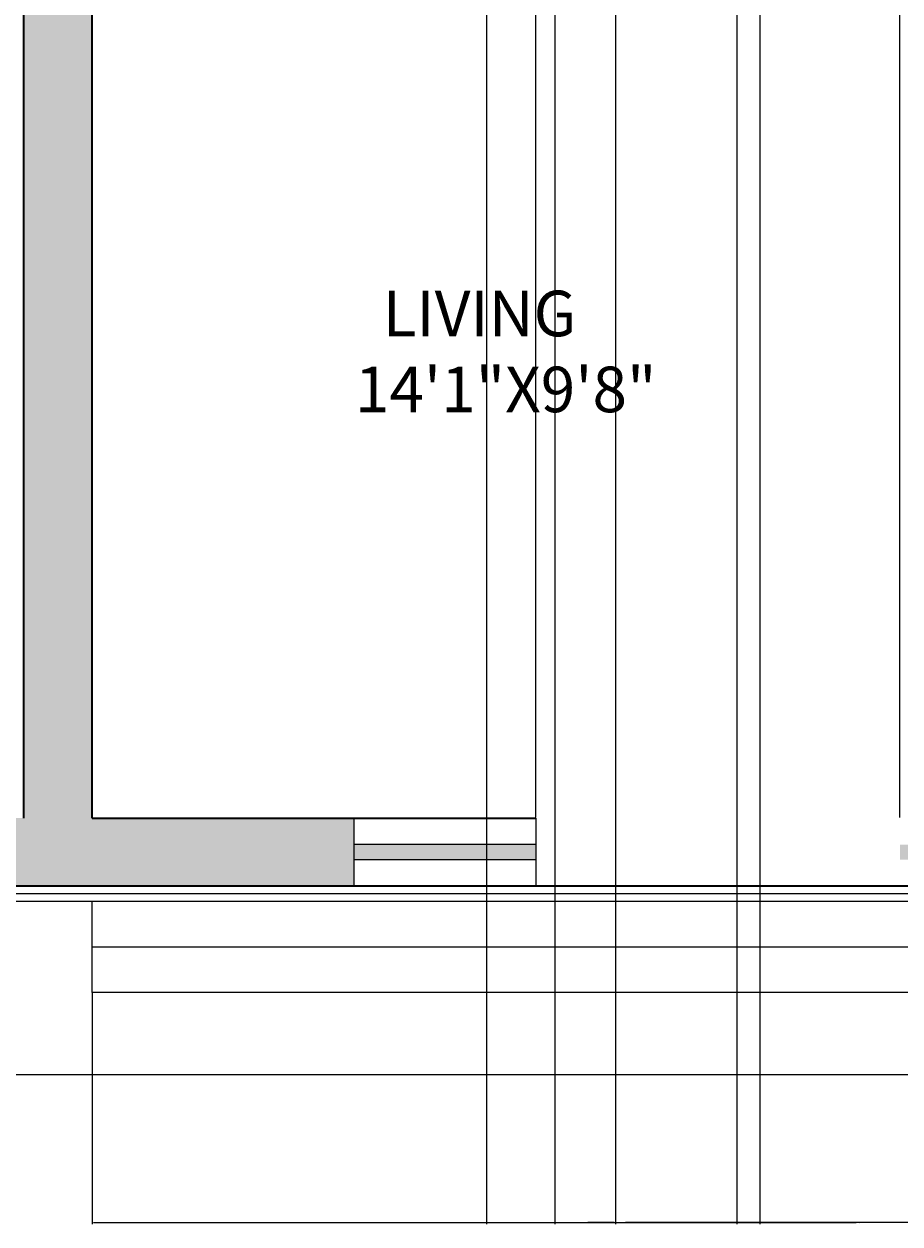
# Model space of a CAD drawing. Units: inches. Extents: x 311 to 815, y -527 to 136.
# Tile 9 of 21: x 539 to 655, y -527 to -368. Entities that reach past the tile are written whole.
import ezdxf

# ---------------------------------------------------------------- set-up
doc = ezdxf.new("R2010")
doc.units = ezdxf.units.IN
doc.header["$MEASUREMENT"] = 0
for name, color, linetype, lineweight in [('A-ANNO-DIMS', 1, 'Continuous', 18), ('A-ANNO-TTLB', 1, 'Continuous', 25), ('A-AREA-IDEN', 8, 'Continuous', 18), ('A-FLOR-EDGE', 1, 'Continuous', 18), ('A-FLOR-STRS', 1, 'Continuous', 18), ('A-GLAZ-PATT', 5, 'Continuous', 13), ('A-WALL-PATT', 242, 'Continuous', 13), ('wall', 1, 'Continuous', 35), ('win', 5, 'Continuous', 18)]:
    doc.layers.add(name, color=color, linetype=linetype, lineweight=lineweight)
doc.styles.get("Standard").update_dxf_attribs({"font": 'arial.ttf'})
doc.dimstyles.get("Standard").update_dxf_attribs({"dimtxt": 0.18, "dimasz": 0.18, "dimexe": 0.18, "dimexo": 0.0625, "dimgap": 0.09, "dimtad": 0, "dimtih": 1, "dimtoh": 1, "dimdec": 1, "dimzin": 0, "dimdsep": 46, "dimlunit": 4, "dimtxsty": 'Standard', "dimcen": 0.09, "dimadec": 0, "dimazin": 0, "dimtfac": 1, "dimtdec": 1, "dimtofl": 0, "dimtmove": 0, "dimatfit": 3, "dimfxl": 1, "dimtolj": 1, "dimtzin": 0, "dimarcsym": 0})

# ---------------------------------------------------------------- blocks, each defined once
blk = doc.blocks.new('WIN-24IN')
for p, q in [((9, 24), (0, 24)), ((3.5, 0), (3.5, 24)), ((5.5, 0), (5.5, 24)), ((9, 0), (0, 0))]:
    blk.add_line(p, q)
blk = doc.blocks.new('*D23')
at = {"layer": 'A-ANNO-DIMS', "color": 0, "lineweight": -2, "transparency": 16777216}
for p, q in [((548.32, -496.19), (548.32, -526.66)), ((722.33, -496.19), (722.33, -526.66)), ((548.5, -526.48), (634.94, -526.48)), ((722.15, -526.48), (635.72, -526.48))]:
    blk.add_line(p, q, dxfattribs=at)
at = {"layer": 'A-ANNO-DIMS', "color": 0, "transparency": 16777216}
for points in [[(548.5, -526.45), (548.5, -526.51), (548.32, -526.48)], [(722.15, -526.45), (722.15, -526.51), (722.33, -526.48)]]:
    blk.add_solid(points, dxfattribs=at)
at = {"layer": 'Defpoints', "color": 0, "transparency": 16777216}
for p in [(548.32, -496.13), (722.33, -496.13), (722.33, -526.48)]:
    blk.add_point(p, dxfattribs=at)
at = {"layer": 'A-ANNO-DIMS', "color": 0, "transparency": 16777216, "insert": (635.33, -526.48), "char_height": 0.18, "attachment_point": 5}
blk.add_mtext('\\A1;14\'-6"', dxfattribs=at)
blk = doc.blocks.new('*D25')
at = {"layer": 'A-ANNO-DIMS', "color": 0, "lineweight": -2, "transparency": 16777216}
for p, q in [((606.82, -473.07), (606.82, 54.4)), ((607, 54.22), (630.49, 54.22)), ((654.64, 54.22), (631.16, 54.22)), ((654.82, -473.07), (654.82, 54.4))]:
    blk.add_line(p, q, dxfattribs=at)
at = {"layer": 'A-ANNO-DIMS', "color": 0, "transparency": 16777216}
for points in [[(607, 54.25), (607, 54.19), (606.82, 54.22)], [(654.64, 54.25), (654.64, 54.19), (654.82, 54.22)]]:
    blk.add_solid(points, dxfattribs=at)
at = {"layer": 'Defpoints', "color": 0, "transparency": 16777216}
for p in [(654.82, 54.22), (606.82, -473.13), (654.82, -473.13)]:
    blk.add_point(p, dxfattribs=at)
at = {"layer": 'A-ANNO-DIMS', "color": 0, "transparency": 16777216, "insert": (630.82, 54.22), "char_height": 0.18, "attachment_point": 5}
blk.add_mtext('\\A1;4\'-0"', dxfattribs=at)
blk = doc.blocks.new('*D27')
at = {"layer": 'A-ANNO-DIMS', "color": 0, "lineweight": -2, "transparency": 16777216}
for p, q in [((548.32, -473.07), (548.32, 54.4)), ((548.5, 54.22), (576.96, 54.22)), ((606.64, 54.22), (578.19, 54.22)), ((606.82, -473.07), (606.82, 54.4))]:
    blk.add_line(p, q, dxfattribs=at)
at = {"layer": 'A-ANNO-DIMS', "color": 0, "transparency": 16777216}
for points in [[(548.5, 54.25), (548.5, 54.19), (548.32, 54.22)], [(606.64, 54.25), (606.64, 54.19), (606.82, 54.22)]]:
    blk.add_solid(points, dxfattribs=at)
at = {"layer": 'Defpoints', "color": 0, "transparency": 16777216}
for p in [(606.82, 54.22), (548.32, -473.13), (606.82, -473.13)]:
    blk.add_point(p, dxfattribs=at)
at = {"layer": 'A-ANNO-DIMS', "color": 0, "transparency": 16777216, "insert": (577.57, 54.22), "char_height": 0.18, "attachment_point": 5}
blk.add_mtext('\\A1;4\'-10 1/2"', dxfattribs=at)
blk = doc.blocks.new('*D34')
at = {"layer": 'A-ANNO-DIMS', "color": 0, "lineweight": -2, "transparency": 16777216}
for p, q in [((609.32, -274.69), (609.32, -526.66)), ((617.32, -274.69), (617.32, -526.66)), ((609.5, -526.48), (612.99, -526.48)), ((617.14, -526.48), (613.65, -526.48))]:
    blk.add_line(p, q, dxfattribs=at)
at = {"layer": 'A-ANNO-DIMS', "color": 0, "transparency": 16777216}
for points in [[(609.5, -526.45), (609.5, -526.51), (609.32, -526.48)], [(617.14, -526.45), (617.14, -526.51), (617.32, -526.48)]]:
    blk.add_solid(points, dxfattribs=at)
at = {"layer": 'Defpoints', "color": 0, "transparency": 16777216}
for p in [(609.32, -274.63), (617.32, -274.63), (617.32, -526.48)]:
    blk.add_point(p, dxfattribs=at)
at = {"layer": 'A-ANNO-DIMS', "color": 0, "transparency": 16777216, "insert": (613.32, -526.48), "char_height": 0.18, "attachment_point": 5}
blk.add_mtext('\\A1;0\'-8"', dxfattribs=at)
blk = doc.blocks.new('*D37')
at = {"layer": 'A-ANNO-DIMS', "color": 0, "lineweight": -2, "transparency": 16777216}
for p, q in [((633.32, -348.19), (633.32, -526.66)), ((665.32, -348.19), (665.32, -526.66)), ((633.5, -526.48), (648.99, -526.48)), ((665.14, -526.48), (649.65, -526.48))]:
    blk.add_line(p, q, dxfattribs=at)
at = {"layer": 'A-ANNO-DIMS', "color": 0, "transparency": 16777216}
for points in [[(633.5, -526.45), (633.5, -526.51), (633.32, -526.48)], [(665.14, -526.45), (665.14, -526.51), (665.32, -526.48)]]:
    blk.add_solid(points, dxfattribs=at)
at = {"layer": 'Defpoints', "color": 0, "transparency": 16777216}
for p in [(633.32, -348.13), (665.32, -348.13), (665.32, -526.48)]:
    blk.add_point(p, dxfattribs=at)
at = {"layer": 'A-ANNO-DIMS', "color": 0, "transparency": 16777216, "insert": (649.32, -526.48), "char_height": 0.18, "attachment_point": 5}
blk.add_mtext('\\A1;2\'-8"', dxfattribs=at)
blk = doc.blocks.new('*D49')
at = {"layer": 'A-ANNO-DIMS', "color": 0, "lineweight": -2, "transparency": 16777216}
for p, q in [((600.32, -112.19), (600.32, -526.66)), ((636.32, -112.19), (636.32, -526.66)), ((600.5, -526.48), (617.99, -526.48)), ((636.14, -526.48), (618.65, -526.48))]:
    blk.add_line(p, q, dxfattribs=at)
at = {"layer": 'A-ANNO-DIMS', "color": 0, "transparency": 16777216}
for points in [[(600.5, -526.45), (600.5, -526.51), (600.32, -526.48)], [(636.14, -526.45), (636.14, -526.51), (636.32, -526.48)]]:
    blk.add_solid(points, dxfattribs=at)
at = {"layer": 'Defpoints', "color": 0, "transparency": 16777216}
for p in [(600.32, -112.13), (636.32, -112.13), (636.32, -526.48)]:
    blk.add_point(p, dxfattribs=at)
at = {"layer": 'A-ANNO-DIMS', "color": 0, "transparency": 16777216, "insert": (618.32, -526.48), "char_height": 0.18, "attachment_point": 5}
blk.add_mtext('\\A1;3\'-0"', dxfattribs=at)

msp = doc.modelspace()

# ---------------------------------------------------------------- hatches: boundary and pattern name
at = {"layer": 'A-GLAZ-PATT'}
h = msp.add_hatch(color=256, dxfattribs=at)
h.dxf.hatch_style = 1
h.paths.add_polyline_path([(415.82, -202.13), (413.82, -202.13), (413.82, -262.13), (415.82, -262.13)])
h.paths.add_polyline_path([(415.82, -390.84), (413.82, -390.84), (413.82, -450.84), (415.82, -450.84)])
h.paths.add_polyline_path([(415.82, -311.57), (413.82, -311.57), (413.82, -335.57), (415.82, -335.57)])
h.paths.add_polyline_path([(509.32, -476.63), (449.32, -476.63), (449.32, -478.63), (509.32, -478.63)])
h.paths.add_polyline_path([(606.82, -476.63), (582.82, -476.63), (582.82, -478.63), (606.82, -478.63)])
h.paths.add_polyline_path([(678.82, -476.63), (654.82, -476.63), (654.82, -478.63), (678.82, -478.63)])
h.paths.add_polyline_path([(718.82, -385.13), (716.82, -385.13), (716.82, -445.13), (718.82, -445.13)])
h.paths.add_polyline_path([(718.82, -262.63), (716.82, -262.63), (716.82, -322.63), (718.82, -322.63)])
h.paths.add_polyline_path([(718.82, -140.13), (716.82, -140.13), (716.82, -200.13), (718.82, -200.13)])
h.paths.add_polyline_path([(718.82, -18.13), (716.82, -18.13), (716.82, -42.13), (718.82, -42.13)])
h.paths.add_polyline_path([(686.82, 18.37), (626.82, 18.37), (626.82, 16.37), (686.82, 16.37)])
h.paths.add_polyline_path([(581.82, 18.37), (557.82, 18.37), (557.82, 16.37), (581.82, 16.37)])
h.paths.add_polyline_path([(509.32, 18.37), (449.32, 18.37), (449.32, 16.37), (509.32, 16.37)])
at = {"layer": 'A-WALL-PATT'}
h = msp.add_hatch(color=256, dxfattribs=at)
h.dxf.hatch_style = 1
h.paths.add_polyline_path([(557.82, 21.87), (509.32, 21.87), (509.32, 12.87), (539.32, 12.87), (539.32, -112.13), (548.32, -112.13), (548.32, -58.63), (557.82, -58.63), (557.82, -49.63), (548.32, -49.63), (548.32, 12.87), (557.82, 12.87)])
h.paths.add_polyline_path([(449.32, 21.87), (410.32, 21.87), (410.32, -15.13), (419.32, -15.13), (419.32, 12.87), (449.32, 12.87)])
h.paths.add_polyline_path([(626.82, 21.87), (581.82, 21.87), (581.82, 12.87), (591.32, 12.87), (591.32, -49.63), (581.82, -49.63), (581.82, -58.63), (591.32, -58.63), (591.32, -112.13), (600.32, -112.13), (600.32, 12.87), (626.82, 12.87)])
h.paths.add_polyline_path([(722.32, 21.87), (686.82, 21.87), (686.82, 12.87), (713.32, 12.87), (713.32, -18.13), (722.32, -18.13)])
h.paths.add_polyline_path([(722.32, -42.13), (713.32, -42.13), (713.32, -73.13), (722.32, -73.13)])
h.paths.add_polyline_path([(501.32, -103.13), (419.32, -103.13), (419.32, -75.13), (410.32, -75.13), (410.32, -126.63), (419.32, -126.63), (419.32, -112.13), (492.32, -112.13), (492.32, -143.13), (501.32, -143.13)])
h.paths.add_polyline_path([(548.32, -165.13), (419.32, -165.13), (419.32, -150.63), (410.32, -150.63), (410.32, -202.13), (419.32, -202.13), (419.32, -174.13), (548.32, -174.13)])
h.paths.add_polyline_path([(722.32, -103.13), (636.32, -103.13), (636.32, -112.13), (713.32, -112.13), (713.32, -140.13), (722.32, -140.13)])
h.paths.add_polyline_path([(548.32, -210.13), (539.32, -210.13), (539.32, -290.13), (419.32, -290.13), (419.32, -262.13), (410.32, -262.13), (410.32, -311.57), (419.32, -311.57), (419.32, -299.13), (469.32, -299.13), (469.32, -348.13), (443.32, -348.13), (443.32, -357.13), (478.32, -357.13), (478.32, -299.13), (548.32, -299.13)])
h.paths.add_polyline_path([(722.32, -200.13), (713.32, -200.13), (713.32, -228.13), (609.32, -228.13), (609.32, -237.13), (713.32, -237.13), (713.32, -262.63), (722.32, -262.63)])
h.paths.add_polyline_path([(722.32, -322.63), (713.32, -322.63), (713.32, -348.13), (633.32, -348.13), (633.32, -357.13), (713.32, -357.13), (713.32, -385.13), (722.32, -385.13)])
h.paths.add_polyline_path([(419.32, -335.57), (410.32, -335.57), (410.32, -390.84), (419.32, -390.84)])
h.paths.add_polyline_path([(419.32, -450.84), (410.32, -450.84), (410.32, -482.13), (449.32, -482.13), (449.32, -473.13), (419.32, -473.13)])
h.paths.add_polyline_path([(582.82, -473.13), (548.32, -473.13), (548.32, -348.13), (539.32, -348.13), (539.32, -473.13), (509.32, -473.13), (509.32, -482.13), (582.82, -482.13)])
h.paths.add_polyline_path([(722.32, -445.13), (713.32, -445.13), (713.32, -473.13), (678.82, -473.13), (678.82, -482.13), (722.32, -482.13)])

# ---------------------------------------------------------------- linework, layer by layer
at = {"layer": 'A-ANNO-TTLB'}
msp.add_lwpolyline([(310.67, 136.01), (815.43, 136.01), (815.43, -506.97), (310.67, -506.97)], close=True, dxfattribs=at)
at = {"layer": 'A-FLOR-EDGE'}
for p, q in [((724.32, -484.13), (408.32, -484.13)), ((723.32, -483.13), (409.32, -483.13))]:
    msp.add_line(p, q, dxfattribs=at)
at = {"layer": 'A-FLOR-STRS'}
for p, q in [((548.32, -496.13), (548.32, -484.13)), ((548.32, -490.13), (722.33, -490.13)), ((722.33, -496.13), (548.32, -496.13))]:
    msp.add_line(p, q, dxfattribs=at)
at = {"layer": 'wall'}
for p, q in [((539.32, -473.13), (539.32, -348.13)), ((548.32, -473.13), (548.32, -348.13)), ((548.32, -473.13), (606.82, -473.13)), ((722.32, -482.13), (410.32, -482.13))]:
    msp.add_line(p, q, dxfattribs=at)

# ---------------------------------------------------------------- block references
at = {"layer": 'win', "rotation": 90.00000000000003}
msp.add_blockref('WIN-24IN', (606.82, -482.13), dxfattribs=at)

# ---------------------------------------------------------------- texts
at = {"layer": 'A-AREA-IDEN', "insert": (582.95, -403.6), "char_height": 6.0073, "attachment_point": 1}
msp.add_mtext_dynamic_manual_height_columns('  LIVING      14\'1"X9\'8"', width=40.6635, gutter_width=1, heights=[0], dxfattribs=at)

# ---------------------------------------------------------------- dimensions: what is measured, and where the dimension line sits
at = {"layer": 'A-ANNO-DIMS'}
for base, p1, p2, picture, middle in [((606.82, 54.22), (548.32, -473.13), (606.82, -473.13), '*D27', (577.57, 54.22)), ((654.82, 54.22), (606.82, -473.13), (654.82, -473.13), '*D25', (630.82, 54.22)), ((636.32, -526.48), (600.32, -112.13), (636.32, -112.13), '*D49', (618.32, -526.48)), ((617.32, -526.48), (609.32, -274.63), (617.32, -274.63), '*D34', (613.32, -526.48)), ((665.32, -526.48), (633.32, -348.13), (665.32, -348.13), '*D37', (649.32, -526.48)), ((722.33, -526.48), (548.32, -496.13), (722.33, -496.13), '*D23', (635.33, -526.48))]:
    dim = msp.add_linear_dim(base=base, p1=p1, p2=p2, dimstyle='Standard', override={"dimdec": 1, "dimlfac": 1, "dimrnd": 0, "dimzin": 1, "dimdsep": 46, "dimlunit": 4, "dimfrac": 2}, dxfattribs=at)
    dim.commit()
    dim.dimension.update_dxf_attribs({"geometry": picture, "text_midpoint": middle})

doc.saveas('drawing.dxf')
